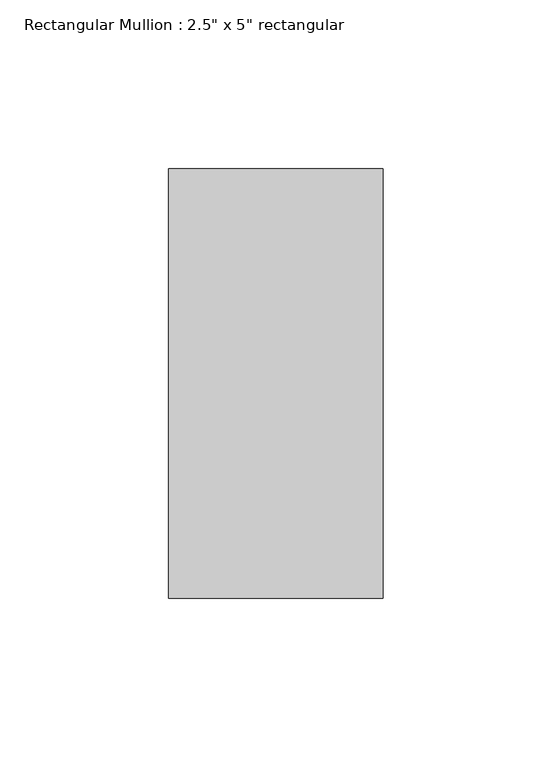
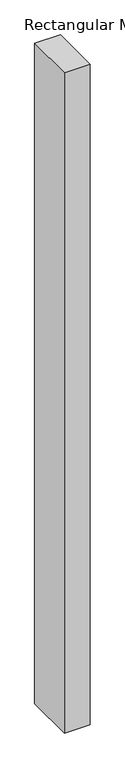
"""IFC4 building model written with IfcOpenShell, lengths in millimetres: member geometry."""

from ifc_helpers import new_model, si_unit, frame, origin, place, context, project, spatial, polyline, outline, extrude, source, transform, mapped, element, save


def member_814d5477(model_context):
    return source(origin(), model_context, "Body", "SweptSolid", [
        extrude(outline(polyline([(31.75, 63.5), (31.75, -63.5), (-31.75, -63.5), (-31.75, 63.5), (31.75, 63.5)])), frame((0.0, 0.0, -1726.8137367), z_axis=(0.0, 0.0, 1.0), x_axis=(1.0, 0.0, 0.0)), (0.0, 0.0, 1.0), 1726.8137367),
    ])


if __name__ == "__main__":
    model = new_model("IFC4")
    model_context = context("Model", 3, world=origin())
    ifc_project = project(units=[si_unit("LENGTHUNIT", "METRE", prefix="MILLI")], contexts=[model_context])
    site = spatial("IfcSite", under=ifc_project)
    building = spatial("IfcBuilding", under=site)
    placement = place(None, origin())
    member_shape = member_814d5477(model_context)
    element("IfcMember", 1, ObjectType="Rectangular Mullion : 2.5\" x 5\" rectangular", at=placement, inside=building, context=model_context, shape_type="MappedRepresentation", body=[
        mapped(member_shape, transform((0.0, 0.0, 0.0), x_axis=(1.0, 0.0, 0.0), y_axis=(0.0, 1.0, 0.0), z_axis=(0.0, 0.0, 1.0))),
    ])
    save(model, "model.ifc")

# Revit data of these elements
# Type "Rectangular Mullion : 2.5\" x 5\" rectangular"
#   built-in parameter 1007304 = 0.416667 (stored number, unit not read)
#   built-in parameter 1007301 = 0.104167 (stored number, unit not read)
#   built-in parameter 1007300 = 0.104167 (stored number, unit not read)
# Element 1 (IfcMember, "Rectangular Mullion : 2.5\" x 5\" rectangular")
#   Materials on its faces: "Aluminum"
# Materials
#   "Aluminum": class "Metal", colour RGB 247 247 247, transparency 0, Description = "Aluminum 6061", Cost = 0
